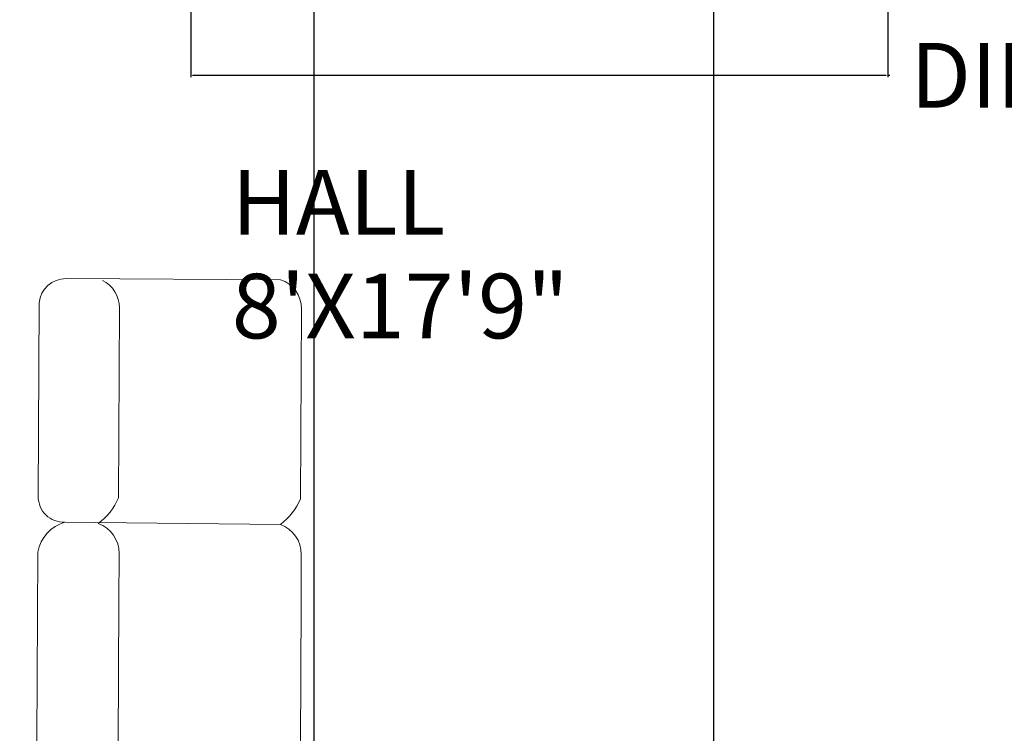
# Model space of a CAD drawing. Units: inches. Extents: x -26 to 575, y -18 to 513.
# Tile 5 of 28: x 31 to 122, y 191 to 257. Entities that reach past the tile are written whole.
import ezdxf

# ---------------------------------------------------------------- set-up
doc = ezdxf.new("R2010")
doc.units = ezdxf.units.IN
doc.header["$MEASUREMENT"] = 0
for name, color, linetype, lineweight in [('A-ANNO-DIMS', 2, 'Continuous', 18), ('A-AREA-IDEN', 7, 'Continuous', 18), ('Furniture', 8, 'Continuous', 15)]:
    doc.layers.add(name, color=color, linetype=linetype, lineweight=lineweight)
doc.styles.get("Standard").update_dxf_attribs({"font": 'arial.ttf', "height": 6})
doc.dimstyles.get("Standard").update_dxf_attribs({"dimtxt": 6, "dimasz": 0.18, "dimexe": 0.18, "dimexo": 0.0625, "dimgap": 0.09, "dimtad": 0, "dimtih": 1, "dimtoh": 1, "dimzin": 0, "dimdsep": 46, "dimlunit": 3, "dimtxsty": 'Standard', "dimcen": 0.09, "dimadec": 0, "dimazin": 0, "dimtfac": 1, "dimtofl": 0, "dimtmove": 0, "dimatfit": 3, "dimfxl": 1, "dimtolj": 1, "dimtzin": 0, "dimarcsym": 0})

# ---------------------------------------------------------------- blocks, each defined once
blk = doc.blocks.new('SOFA-L-SECTIONAL')
for p, q in [((22.738, 97.988, -13.498), (2.817, 98.09, -13.498)), ((0.328, 95.831, -13.498), (0.235, 77.862, -13.498)), ((7.684, 77.72, -13.498), (7.775, 95.38, -13.498)), ((24.594, 77.633, -13.498), (24.685, 95.292, -13.498)), ((2.7, 75.474, -13.498), (22.724, 75.267, -13.498)), ((0.208, 72.698, -13.498), (0.118, 55.245, -13.498)), ((7.737, 68.115, -13.498), (7.76, 72.556, -13.498)), ((24.648, 68.028, -13.498), (24.671, 72.469, -13.498)), ((7.669, 54.896, -13.498), (7.737, 68.115, -13.498)), ((24.58, 54.809, -13.498), (24.648, 68.028, -13.498)), ((2.375, 52.548, -13.498), (22.194, 52.446, -13.498)), ((22.503, 52.449, -13.498), (2.582, 52.551, -13.498)), ((0.093, 50.292, -13.498), (0, 32.323, -13.498)), ((7.449, 32.181, -13.498), (7.54, 49.841, -13.498)), ((24.36, 32.094, -13.498), (24.451, 49.754, -13.498)), ((2.465, 29.935, -13.498), (22.489, 29.728, -13.498)), ((51.416, 24.36, -13.498), (33.756, 24.451, -13.498)), ((31.061, 22.504, -13.498), (30.958, 2.582, -13.498)), ((53.782, 22.49, -13.498), (53.575, 2.465, -13.498)), ((28.5, 7.133, -13.498), (28.258, 7.134, -13.498)), ((51.327, 7.05, -13.498), (33.667, 7.141, -13.498)), ((30.972, 5.194, -13.498), (30.972, 5.123, -13.498)), ((33.218, 0.093, -13.498), (51.187, 0, -13.498))]:
    blk.add_line(p, q)
for centre, radius, start, end in [((2.804, 95.604, -13.498), 2.487, 89.70451, 174.75427), ((4.956, 95.394, -13.498), 2.819, 359.70451, 63.77883), ((21.867, 95.307, -13.498), 2.819, 359.70451, 71.99328), ((2.612, 77.849, -13.498), 2.377, 179.70451, 272.11333), ((2.36, 80.007, -13.498), 5.794, 306.58832, 336.75474), ((19.27, 79.92, -13.498), 5.794, 306.58832, 336.75474), ((3.665, 72.101, -13.498), 3.508, 105.97251, 170.1982), ((4.797, 72.571, -13.498), 2.963, 359.70451, 69.94564), ((21.708, 72.484, -13.498), 2.963, 359.70451, 69.94564), ((2.841, 55.231, -13.498), 2.723, 179.70451, 260.14867), ((5.295, 54.907, -13.498), 2.374, 286.46225, 359.73347), ((22.206, 54.82, -13.498), 2.374, 269.70451, 359.73347), ((2.569, 50.065, -13.498), 2.487, 89.70451, 174.75427), ((4.721, 49.855, -13.498), 2.819, 359.70451, 63.77883), ((21.632, 49.768, -13.498), 2.819, 359.70451, 71.99328), ((2.377, 32.311, -13.498), 2.377, 179.70451, 272.11333), ((2.125, 34.468, -13.498), 5.794, 306.58832, 336.75474), ((19.036, 34.381, -13.498), 5.794, 306.58832, 336.75474), ((3.602, 26.521, -13.498), 3.601, 357.71664, 177.71664), ((23.889, 22.801, -13.498), 7.123, 359.70451, 100.30514), ((28.369, 28.51, -13.498), 21.376, 182.62045, 269.70451), ((28.369, 28.51, -13.498), 28.423, 183.69155, 269.65279), ((33.742, 21.632, -13.498), 2.819, 89.70451, 161.99328), ((49.129, 19.036, -13.498), 5.794, 36.58832, 66.75474), ((27.431, 3.649, -13.498), 3.644, 282.13059, 72.938), ((33.653, 4.323, -13.498), 2.819, 89.70451, 161.99328), ((49.04, 1.726, -13.498), 5.794, 36.58832, 66.75474), ((33.445, 2.569, -13.498), 2.487, 179.70451, 264.75427), ((51.199, 2.378, -13.498), 2.377, 269.70451, 2.11333)]:
    blk.add_arc(centre, radius, start, end)
blk = doc.blocks.new('*D24')
at = {"layer": 'A-ANNO-DIMS', "color": 0, "lineweight": -2, "transparency": 16777216}
for p, q in [((46.82, 261.725), (46.82, 251.899)), ((111.544, 261.725), (111.544, 251.899)), ((47, 252.079), (111.364, 252.079)), ((111.544, 252.079), (111.724, 252.079))]:
    blk.add_line(p, q, dxfattribs=at)
at = {"layer": 'A-ANNO-DIMS', "color": 0, "transparency": 16777216}
for points in [[(47, 252.109), (47, 252.049), (46.82, 252.079)], [(111.364, 252.109), (111.364, 252.049), (111.544, 252.079)]]:
    blk.add_solid(points, dxfattribs=at)
at = {"layer": 'Defpoints', "color": 0, "transparency": 16777216}
for p in [(46.82, 261.787), (111.544, 261.787), (111.544, 252.079)]:
    blk.add_point(p, dxfattribs=at)
at = {"layer": 'A-ANNO-DIMS', "color": 0, "transparency": 16777216, "insert": (162.09, 252.079), "char_height": 6, "attachment_point": 5}
blk.add_mtext('\\A1;DINING SET 5\'-4 1/2" TYP.', dxfattribs=at)
blk = doc.blocks.new('*D28')
at = {"layer": 'A-ANNO-DIMS', "color": 0, "lineweight": -2, "transparency": 16777216}
for p, q in [((58.224, 466.445), (58.224, -8.972)), ((95.349, 466.445), (95.349, -8.972)), ((58.404, -8.792), (68.723, -8.792)), ((95.169, -8.792), (84.849, -8.792))]:
    blk.add_line(p, q, dxfattribs=at)
at = {"layer": 'A-ANNO-DIMS', "color": 0, "transparency": 16777216}
for points in [[(58.404, -8.762), (58.404, -8.822), (58.224, -8.792)], [(95.169, -8.762), (95.169, -8.822), (95.349, -8.792)]]:
    blk.add_solid(points, dxfattribs=at)
at = {"layer": 'Defpoints', "color": 0, "transparency": 16777216}
for p in [(58.224, 466.508), (95.349, 466.508), (95.349, -8.792)]:
    blk.add_point(p, dxfattribs=at)
at = {"layer": 'A-ANNO-DIMS', "color": 0, "transparency": 16777216, "insert": (76.786, -8.792), "char_height": 6, "attachment_point": 5}
blk.add_mtext('\\A1;3\'-1"', dxfattribs=at)
blk = doc.blocks.new('*D50')
at = {"layer": 'A-ANNO-DIMS', "color": 0, "lineweight": -2, "transparency": 16777216}
for p, q in [((27.177, 466.445), (27.177, -8.972)), ((58.224, 466.445), (58.224, -8.972)), ((27.357, -8.792), (34.584, -8.792)), ((58.044, -8.792), (50.816, -8.792))]:
    blk.add_line(p, q, dxfattribs=at)
at = {"layer": 'A-ANNO-DIMS', "color": 0, "transparency": 16777216}
for points in [[(27.357, -8.762), (27.357, -8.822), (27.177, -8.792)], [(58.044, -8.762), (58.044, -8.822), (58.224, -8.792)]]:
    blk.add_solid(points, dxfattribs=at)
at = {"layer": 'Defpoints', "color": 0, "transparency": 16777216}
for p in [(27.177, 466.508), (58.224, 466.508), (58.224, -8.792)]:
    blk.add_point(p, dxfattribs=at)
at = {"layer": 'A-ANNO-DIMS', "color": 0, "transparency": 16777216, "insert": (42.7, -8.792), "char_height": 6, "attachment_point": 5}
blk.add_mtext('\\A1;2\'-7"', dxfattribs=at)

msp = doc.modelspace()

# ---------------------------------------------------------------- block references
at = {"layer": 'Furniture'}
msp.add_blockref('SOFA-L-SECTIONAL', (32.395, 135.109), dxfattribs=at)

# ---------------------------------------------------------------- texts
at = {"layer": 'A-AREA-IDEN'}
for s, p in [('HALL', (50.611, 237.292)), ('8\'X17\'9"', (50.612, 227.653))]:
    msp.add_text(s, height=6, rotation=0.00167, dxfattribs=at).set_placement(p)

# ---------------------------------------------------------------- dimensions: what is measured, and where the dimension line sits
at = {"layer": 'A-ANNO-DIMS'}
for base, p1, p2, picture, middle in [((58.224, -8.792), (27.177, 466.508), (58.224, 466.508), '*D50', (42.7, -8.792)), ((95.349, -8.792), (58.224, 466.508), (95.349, 466.508), '*D28', (76.786, -8.792))]:
    dim = msp.add_linear_dim(base=base, p1=p1, p2=p2, dimstyle='Standard', override={"dimdec": 1, "dimlfac": 1, "dimrnd": 0, "dimzin": 1, "dimdsep": 46, "dimlunit": 4, "dimfrac": 2}, dxfattribs=at)
    dim.commit()
    dim.dimension.update_dxf_attribs({"geometry": picture, "text_midpoint": middle})
dim = msp.add_linear_dim(base=(111.544, 252.079), p1=(46.82, 261.787), p2=(111.544, 261.787), text='DINING SET <> TYP.', dimstyle='Standard', override={"dimdec": 1, "dimlfac": 1, "dimrnd": 0, "dimzin": 1, "dimdsep": 46, "dimlunit": 4, "dimfrac": 2}, dxfattribs=at)
dim.commit()
dim.dimension.update_dxf_attribs({"geometry": '*D24', "text_midpoint": (162.09, 252.079)})

doc.saveas('drawing.dxf')
